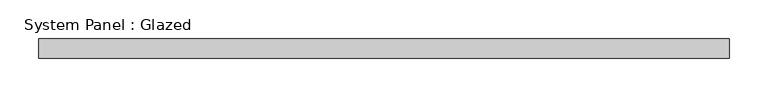
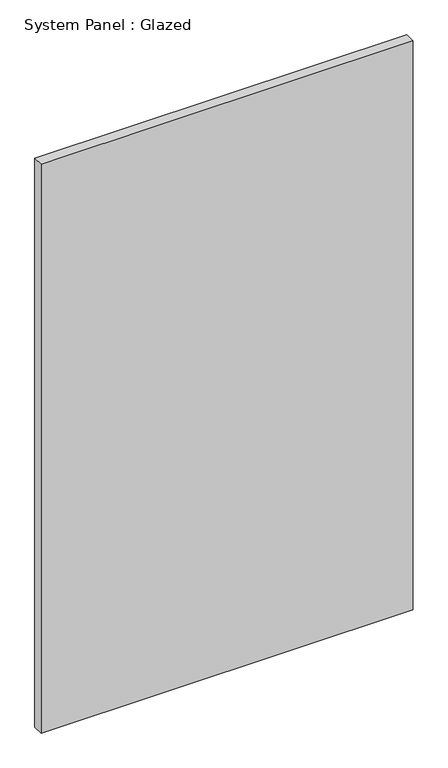
"""IFC4 building model written with IfcOpenShell, lengths in millimetres: plate geometry, System Panel : Glazed."""

from ifc_helpers import new_model, si_unit, origin, origin_with_axes, place, context, project, spatial, polyline, outline, extrude, source, transform, mapped, element, save


def system_panel_glazed_2b1bd5bc(model_context):
    return source(origin(), model_context, "Body", "SweptSolid", [
        extrude(outline(polyline([(447.675, 19.05), (-447.675, 19.05), (-447.675, 44.45), (447.675, 44.45), (447.675, 19.05)])), origin_with_axes(), (0.0, 0.0, 1.0), 1447.1253432),
    ])


if __name__ == "__main__":
    model = new_model("IFC4")
    model_context = context("Model", 3, world=origin())
    ifc_project = project(units=[si_unit("LENGTHUNIT", "METRE", prefix="MILLI")], contexts=[model_context])
    site = spatial("IfcSite", under=ifc_project)
    building = spatial("IfcBuilding", under=site)
    placement = place(None, origin())
    system_panel_glazed_shape = system_panel_glazed_2b1bd5bc(model_context)
    element("IfcPlate", 1, ObjectType="System Panel : Glazed", at=placement, inside=building, context=model_context, shape_type="MappedRepresentation", body=[
        mapped(system_panel_glazed_shape, transform((0.0, 0.0, 0.0), x_axis=(1.0, 0.0, 0.0), y_axis=(0.0, 1.0, 0.0), z_axis=(0.0, 0.0, 1.0))),
    ])
    save(model, "model.ifc")

# Revit data of these elements
# Type "System Panel : Glazed"
#   Construction Type Id = "GSP4R"
#   Analytic Construction = "1/8 in Pilkington single glazing"
#   Visual Light Transmittance = 0.9
#   Solar Heat Gain Coefficient = 0.86
#   Heat Transfer Coefficient (U) = 1.18115 BTU/(h·ft²·°F)
#   Define Thermal Properties by = 1
# Element 1 (IfcPlate, "System Panel : Glazed")
#   Materials on its faces: "Glass"
# Materials
#   "Glass": class "Glass", colour RGB 0 128 192, transparency 0.75, Description = "Soda Lime Glass", Cost = 0
